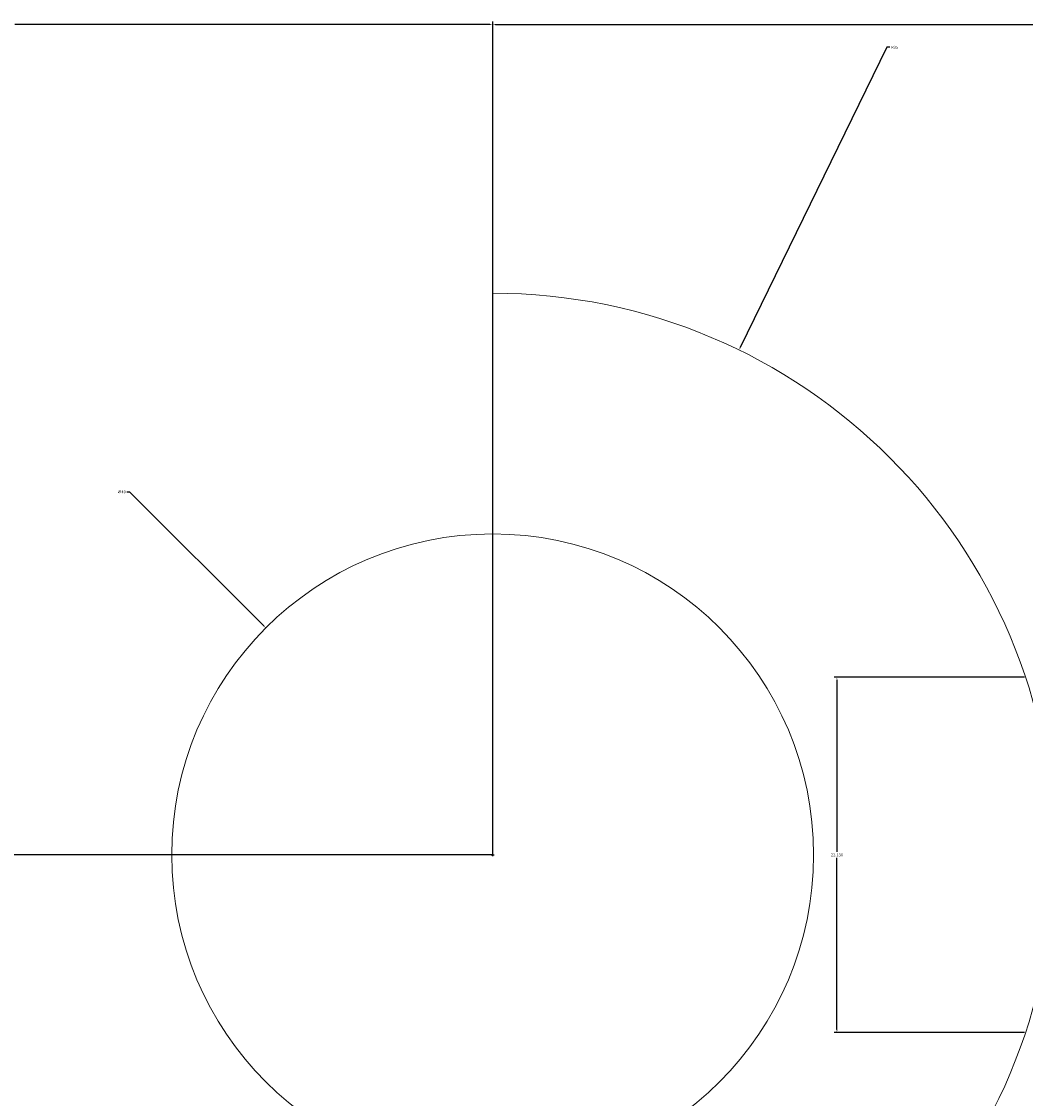
# Model space of a CAD drawing. Units: millimetres. Extents: x 3108 to 3332, y 1482 to 1586.
# Tile 3 of 5: x 3171 to 3233, y 1519 to 1586. Entities that reach past the tile are written whole.
import ezdxf

# ---------------------------------------------------------------- set-up
doc = ezdxf.new("R2010")
doc.units = ezdxf.units.MM
doc.layers.add('M-CONS', color=8, linetype='Continuous', lineweight=18)
doc.layers.add('M-DIMS', color=2, linetype='Continuous', lineweight=18)
doc.styles.get("Standard").update_dxf_attribs({"font": 'arial.ttf'})
doc.dimstyles.get("Standard").update_dxf_attribs({"dimtxt": 0.18, "dimasz": 0.18, "dimexe": 0.18, "dimexo": 0.0625, "dimgap": 0.09, "dimtad": 0, "dimtih": 1, "dimtoh": 1, "dimdec": 4, "dimzin": 0, "dimdsep": 46, "dimtxsty": 'Standard', "dimcen": 0.09, "dimadec": 0, "dimazin": 0, "dimtfac": 1, "dimtdec": 4, "dimtofl": 0, "dimtmove": 0, "dimatfit": 3, "dimfxl": 1, "dimtolj": 1, "dimtzin": 0, "dimarcsym": 0})

# ---------------------------------------------------------------- blocks, each defined once
blk = doc.blocks.new('*D3')
at = {"layer": 'Defpoints', "color": 0, "transparency": 16777216}
for p in [(3319.945, 1585.693), (3319.945, 1573.943), (3199.945, 1568.943)]:
    blk.add_point(p, dxfattribs=at)
at = {"layer": 'M-DIMS', "color": 0, "lineweight": -2, "transparency": 16777216}
for p, q in [((3199.945, 1569.006), (3199.945, 1585.873)), ((3319.945, 1574.006), (3319.945, 1585.873)), ((3200.125, 1585.693), (3259.665, 1585.693)), ((3319.765, 1585.693), (3260.225, 1585.693))]:
    blk.add_line(p, q, dxfattribs=at)
at = {"layer": 'M-DIMS', "color": 0, "transparency": 16777216}
for points in [[(3200.125, 1585.723), (3200.125, 1585.663), (3199.945, 1585.693)], [(3319.765, 1585.723), (3319.765, 1585.663), (3319.945, 1585.693)]]:
    blk.add_solid(points, dxfattribs=at)
at = {"layer": 'M-DIMS', "color": 0, "transparency": 16777216, "insert": (3259.945, 1585.693), "char_height": 0.18, "attachment_point": 5}
blk.add_mtext('\\A1;120', dxfattribs=at)
blk = doc.blocks.new('*D6')
at = {"layer": 'Defpoints', "color": 0, "transparency": 16777216}
for p in [(3199.945, 1585.693), (3139.945, 1568.943), (3199.945, 1533.943)]:
    blk.add_point(p, dxfattribs=at)
at = {"layer": 'M-DIMS', "color": 0, "lineweight": -2, "transparency": 16777216}
for p, q in [((3139.945, 1569.006), (3139.945, 1585.873)), ((3199.945, 1534.006), (3199.945, 1585.873)), ((3140.125, 1585.693), (3169.726, 1585.693)), ((3199.765, 1585.693), (3170.164, 1585.693))]:
    blk.add_line(p, q, dxfattribs=at)
at = {"layer": 'M-DIMS', "color": 0, "transparency": 16777216}
for points in [[(3140.125, 1585.723), (3140.125, 1585.663), (3139.945, 1585.693)], [(3199.765, 1585.723), (3199.765, 1585.663), (3199.945, 1585.693)]]:
    blk.add_solid(points, dxfattribs=at)
at = {"layer": 'M-DIMS', "color": 0, "transparency": 16777216, "insert": (3169.945, 1585.693), "char_height": 0.18, "attachment_point": 5}
blk.add_mtext('\\A1;60', dxfattribs=at)
blk = doc.blocks.new('*D8')
at = {"layer": 'Defpoints', "color": 0, "transparency": 16777216}
for p in [(3221.399, 1545.011), (3233.149, 1545.011), (3233.149, 1522.875)]:
    blk.add_point(p, dxfattribs=at)
at = {"layer": 'M-DIMS', "color": 0, "lineweight": -2, "transparency": 16777216}
for p, q in [((3233.086, 1545.011), (3221.219, 1545.011)), ((3221.399, 1544.831), (3221.399, 1534.125)), ((3221.399, 1523.055), (3221.399, 1533.761)), ((3233.086, 1522.875), (3221.219, 1522.875))]:
    blk.add_line(p, q, dxfattribs=at)
at = {"layer": 'M-DIMS', "color": 0, "transparency": 16777216}
for points in [[(3221.369, 1544.831), (3221.429, 1544.831), (3221.399, 1545.011)], [(3221.369, 1523.055), (3221.429, 1523.055), (3221.399, 1522.875)]]:
    blk.add_solid(points, dxfattribs=at)
at = {"layer": 'M-DIMS', "color": 0, "transparency": 16777216, "insert": (3221.399, 1533.943), "char_height": 0.18, "attachment_point": 5}
blk.add_mtext('\\A1;22.136', dxfattribs=at)
blk = doc.blocks.new('*D9')
at = {"layer": 'Defpoints', "color": 0, "transparency": 16777216}
for p in [(3108.195, 1533.943), (3199.945, 1533.943), (3159.945, 1498.943)]:
    blk.add_point(p, dxfattribs=at)
at = {"layer": 'M-DIMS', "color": 0, "lineweight": -2, "transparency": 16777216}
for p, q in [((3199.882, 1533.943), (3108.015, 1533.943)), ((3108.195, 1533.763), (3108.195, 1516.625)), ((3108.195, 1499.123), (3108.195, 1516.261)), ((3159.882, 1498.943), (3108.015, 1498.943))]:
    blk.add_line(p, q, dxfattribs=at)
at = {"layer": 'M-DIMS', "color": 0, "transparency": 16777216}
for points in [[(3108.165, 1533.763), (3108.225, 1533.763), (3108.195, 1533.943)], [(3108.165, 1499.123), (3108.225, 1499.123), (3108.195, 1498.943)]]:
    blk.add_solid(points, dxfattribs=at)
at = {"layer": 'M-DIMS', "color": 0, "transparency": 16777216, "insert": (3108.195, 1516.443), "char_height": 0.18, "attachment_point": 5}
blk.add_mtext('\\A1;35', dxfattribs=at)
blk = doc.blocks.new('*D12')
at = {"layer": 'Defpoints', "color": 0, "transparency": 16777216}
for p in [(3215.298, 1565.396), (3199.945, 1533.943)]:
    blk.add_point(p, dxfattribs=at)
at = {"layer": 'M-DIMS', "color": 0, "lineweight": -2, "transparency": 16777216}
for p, q in [((3224.51, 1584.268), (3215.377, 1565.558)), ((3224.69, 1584.268), (3224.51, 1584.268)), ((3199.855, 1533.943), (3200.035, 1533.943)), ((3199.945, 1533.853), (3199.945, 1534.033))]:
    blk.add_line(p, q, dxfattribs=at)
at = {"layer": 'M-DIMS', "color": 0, "transparency": 16777216}
blk.add_solid([(3215.35, 1565.571), (3215.404, 1565.544), (3215.298, 1565.396)], dxfattribs=at)
at = {"layer": 'M-DIMS', "color": 0, "transparency": 16777216, "insert": (3224.996, 1584.268), "char_height": 0.18, "attachment_point": 5}
blk.add_mtext('\\A1;R35', dxfattribs=at)
blk = doc.blocks.new('*D14')
at = {"layer": 'Defpoints', "color": 0, "transparency": 16777216}
for p in [(3185.801, 1548.084), (3214.088, 1519.802)]:
    blk.add_point(p, dxfattribs=at)
at = {"layer": 'M-DIMS', "color": 0, "lineweight": -2, "transparency": 16777216}
for p, q in [((3177.135, 1556.568), (3177.315, 1556.568)), ((3177.315, 1556.568), (3185.674, 1548.211)), ((3199.855, 1533.943), (3200.035, 1533.943)), ((3199.945, 1533.853), (3199.945, 1534.033))]:
    blk.add_line(p, q, dxfattribs=at)
at = {"layer": 'M-DIMS', "color": 0, "transparency": 16777216}
blk.add_solid([(3185.695, 1548.232), (3185.653, 1548.19), (3185.801, 1548.084)], dxfattribs=at)
at = {"layer": 'M-DIMS', "color": 0, "transparency": 16777216, "insert": (3176.819, 1556.568), "char_height": 0.18, "attachment_point": 5}
blk.add_mtext('\\A1;∅40', dxfattribs=at)

msp = doc.modelspace()

# ---------------------------------------------------------------- linework, layer by layer
at = {"layer": 'M-CONS'}
msp.add_circle((3199.9448, 1533.9431), 20, dxfattribs=at)
msp.add_arc((3199.9448, 1533.9431), 35, 270, 90, dxfattribs=at)

# ---------------------------------------------------------------- dimensions: what is measured, and where the dimension line sits
at = {"layer": 'M-DIMS'}
for base, p1, p2, picture, middle in [((3199.9448, 1585.6931), (3139.9448, 1568.9431), (3199.9448, 1533.9431), '*D6', (3169.9448, 1585.6931)), ((3319.9448, 1585.6931), (3199.9448, 1568.9431), (3319.9448, 1573.9431), '*D3', (3259.9448, 1585.6931))]:
    dim = msp.add_linear_dim(base=base, p1=p1, p2=p2, dimstyle='Standard', override={"dimdec": 0, "dimlfac": 1, "dimrnd": 0, "dimzin": 0, "dimdsep": 46, "dimlunit": 2}, dxfattribs=at)
    dim.commit()
    dim.dimension.update_dxf_attribs({"geometry": picture, "text_midpoint": middle})
dim = msp.add_radius_dim(center=(3199.9448, 1533.9431), mpoint=(3215.298, 1565.3959), dimstyle='Standard', override={"dimdec": 0, "dimlfac": 1, "dimrnd": 0, "dimzin": 0, "dimdsep": 46, "dimlunit": 2}, dxfattribs=at)
dim.commit()
dim.dimension.update_dxf_attribs({"geometry": '*D12', "text_midpoint": (3224.9957, 1584.2676), "dimtype": 164})
dim = msp.add_diameter_dim_2p(p1=(3214.0883, 1519.8024), p2=(3185.8012, 1548.0838), dimstyle='Standard', override={"dimdec": 0, "dimlfac": 1, "dimrnd": 0, "dimzin": 0, "dimdsep": 46, "dimlunit": 2}, dxfattribs=at)
dim.commit()
dim.dimension.update_dxf_attribs({"geometry": '*D14', "text_midpoint": (3176.8185, 1556.5682), "dimtype": 163})
for base, p1, p2, override, picture, middle in [((3221.3987, 1545.0111), (3233.1487, 1522.8751), (3233.1487, 1545.0111), {"dimdec": 3, "dimlfac": 1, "dimrnd": 0, "dimzin": 0, "dimdsep": 46, "dimlunit": 2}, '*D8', (3221.3987, 1533.9431)), ((3108.1948, 1533.9431), (3159.9448, 1498.9431), (3199.9448, 1533.9431), {"dimdec": 0, "dimlfac": 1, "dimrnd": 0, "dimzin": 0, "dimdsep": 46, "dimlunit": 2}, '*D9', (3108.1948, 1516.4431))]:
    dim = msp.add_linear_dim(base=base, p1=p1, p2=p2, angle=90, dimstyle='Standard', override=override, dxfattribs=at)
    dim.commit()
    dim.dimension.update_dxf_attribs({"geometry": picture, "text_midpoint": middle})

doc.saveas('drawing.dxf')
